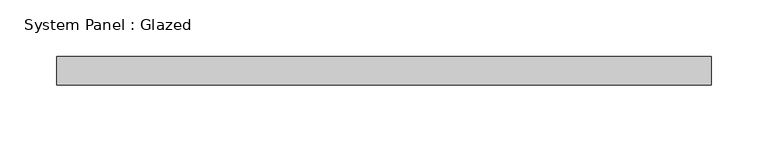
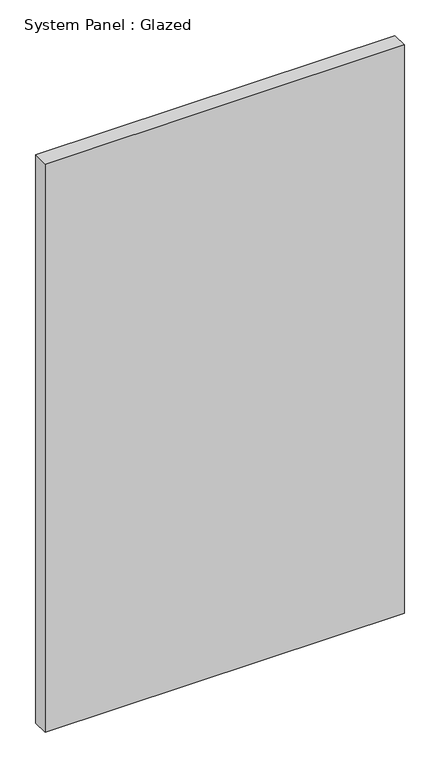
"""IFC4 building model written with IfcOpenShell, lengths in millimetres: plate geometry, System Panel : Glazed."""

from ifc_helpers import new_model, si_unit, origin, origin_with_axes, place, context, project, spatial, polyline, outline, extrude, source, transform, mapped, element, save


def system_panel_glazed_3918bd16(model_context):
    return source(origin(), model_context, "Body", "SweptSolid", [
        extrude(outline(polyline([(288.925, 19.05), (-288.925, 19.05), (-288.925, 44.45), (288.925, 44.45), (288.925, 19.05)])), origin_with_axes(), (0.0, 0.0, 1.0), 965.2),
    ])


if __name__ == "__main__":
    model = new_model("IFC4")
    model_context = context("Model", 3, world=origin())
    ifc_project = project(units=[si_unit("LENGTHUNIT", "METRE", prefix="MILLI")], contexts=[model_context])
    site = spatial("IfcSite", under=ifc_project)
    building = spatial("IfcBuilding", under=site)
    placement = place(None, origin())
    system_panel_glazed_shape = system_panel_glazed_3918bd16(model_context)
    element("IfcPlate", 1, ObjectType="System Panel : Glazed", at=placement, inside=building, context=model_context, shape_type="MappedRepresentation", body=[
        mapped(system_panel_glazed_shape, transform((0.0, 0.0, 0.0), x_axis=(1.0, 0.0, 0.0), y_axis=(0.0, 1.0, 0.0), z_axis=(0.0, 0.0, 1.0))),
    ])
    save(model, "model.ifc")

# Revit data of these elements
# Type "System Panel : Glazed"
#   Construction Type Id = "GSP4R"
#   Analytic Construction = "1/8 in Pilkington single glazing"
#   Visual Light Transmittance = 0.9
#   Solar Heat Gain Coefficient = 0.86
#   Heat Transfer Coefficient (U) = 1.18115 BTU/(h·ft²·°F)
# Element 1 (IfcPlate, "System Panel : Glazed")
#   Materials on its faces: "Glass"
# Materials
#   "Glass": class "Glass", colour RGB 0 128 192, transparency 0.75, Description = "Soda Lime Glass", Cost = 0
